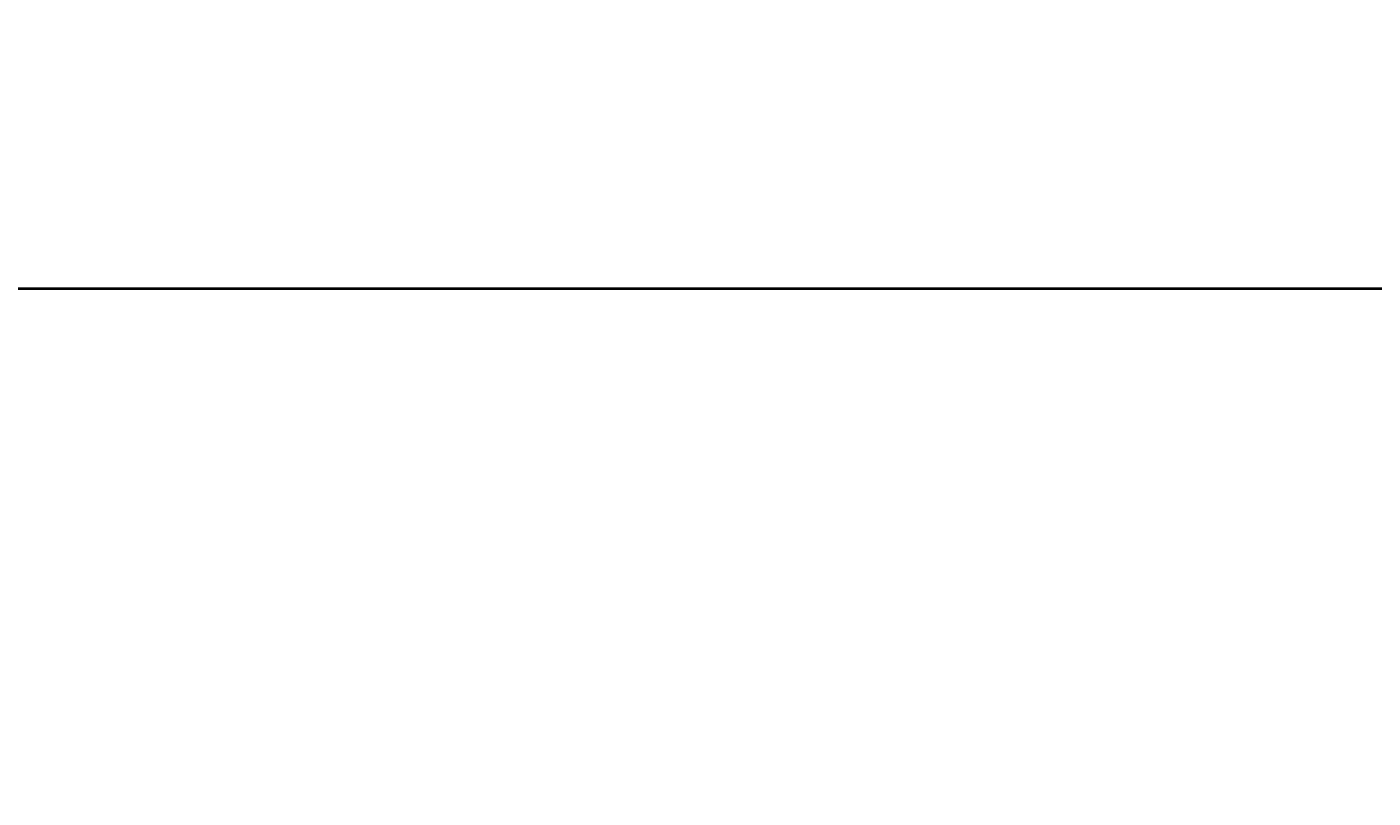
# Model space of a CAD drawing. Units: inches. Extents: x -301 to 715, y -607 to 364.
# Tile 63 of 141: x -93 to -62, y -235 to -218. Entities that reach past the tile are written whole.
import ezdxf

# ---------------------------------------------------------------- set-up
doc = ezdxf.new("R2010")
doc.units = ezdxf.units.IN
doc.header["$MEASUREMENT"] = 0
doc.layers.add('A-ANNO-DIMS', color=2, linetype='Continuous', lineweight=18)
doc.layers.add('A-WALL', color=3, linetype='Continuous', lineweight=40)
doc.styles.get("Standard").update_dxf_attribs({"font": 'arial.ttf'})
doc.dimstyles.get("Standard").update_dxf_attribs({"dimtxt": 0.18, "dimasz": 0.18, "dimexe": 0.18, "dimexo": 0.0625, "dimgap": 0.09, "dimtad": 0, "dimtih": 1, "dimtoh": 1, "dimdec": 1, "dimzin": 0, "dimdsep": 46, "dimlunit": 4, "dimtxsty": 'Standard', "dimcen": 0.09, "dimclrd": 3, "dimclre": 4, "dimclrt": 6, "dimadec": 0, "dimazin": 0, "dimtfac": 1, "dimtdec": 1, "dimtofl": 0, "dimtmove": 0, "dimatfit": 3, "dimfxl": 1, "dimtfill": 2, "dimtfillclr": 51, "dimtolj": 1, "dimtzin": 0, "dimarcsym": 0})

# ---------------------------------------------------------------- blocks, each defined once
blk = doc.blocks.new('*D147')
at = {"layer": 'A-ANNO-DIMS', "color": 4, "lineweight": -2, "transparency": 16777216}
for p, q in [((-103.603, -223.88), (-103.603, -296.865)), ((-45.603, -223.88), (-45.603, -296.865))]:
    blk.add_line(p, q, dxfattribs=at)
at = {"layer": 'A-ANNO-DIMS', "color": 3, "lineweight": -2, "transparency": 16777216}
for p, q in [((-103.423, -296.685), (-75.006, -296.685)), ((-45.783, -296.685), (-74.2, -296.685))]:
    blk.add_line(p, q, dxfattribs=at)
at = {"layer": 'A-ANNO-DIMS', "color": 3, "transparency": 16777216}
for points in [[(-103.423, -296.655), (-103.423, -296.715), (-103.603, -296.685)], [(-45.783, -296.655), (-45.783, -296.715), (-45.603, -296.685)]]:
    blk.add_solid(points, dxfattribs=at)
at = {"layer": 'Defpoints', "color": 0, "transparency": 16777216}
for p in [(-103.603, -223.818), (-45.603, -223.818), (-45.603, -296.685)]:
    blk.add_point(p, dxfattribs=at)
at = {"layer": 'A-ANNO-DIMS', "color": 6, "transparency": 16777216, "insert": (-74.603, -296.685), "char_height": 0.18, "attachment_point": 5, "bg_fill": 1, "box_fill_scale": 1.25, "bg_fill_color": 51, "bg_fill_transparency": 0}
blk.add_mtext('\\A1;4\'-10"', dxfattribs=at)
blk = doc.blocks.new('*D151')
at = {"layer": 'A-ANNO-DIMS', "color": 4, "lineweight": -2, "transparency": 16777216}
for p, q in [((-204.603, -223.755), (-204.603, 359.612)), ((-45.603, -214.755), (-45.603, 359.612))]:
    blk.add_line(p, q, dxfattribs=at)
at = {"layer": 'A-ANNO-DIMS', "color": 3, "lineweight": -2, "transparency": 16777216}
for p, q in [((-204.423, 359.432), (-125.494, 359.432)), ((-45.783, 359.432), (-124.713, 359.432))]:
    blk.add_line(p, q, dxfattribs=at)
at = {"layer": 'A-ANNO-DIMS', "color": 3, "transparency": 16777216}
for points in [[(-204.423, 359.462), (-204.423, 359.402), (-204.603, 359.432)], [(-45.783, 359.462), (-45.783, 359.402), (-45.603, 359.432)]]:
    blk.add_solid(points, dxfattribs=at)
at = {"layer": 'Defpoints', "color": 0, "transparency": 16777216}
for p in [(-45.603, 359.432), (-45.603, -214.818), (-204.603, -223.818)]:
    blk.add_point(p, dxfattribs=at)
at = {"layer": 'A-ANNO-DIMS', "color": 6, "transparency": 16777216, "insert": (-125.103, 359.432), "char_height": 0.18, "attachment_point": 5, "bg_fill": 1, "box_fill_scale": 1.25, "bg_fill_color": 51, "bg_fill_transparency": 0}
blk.add_mtext('\\A1;13\'-3"', dxfattribs=at)
blk = doc.blocks.new('*D158')
at = {"layer": 'A-ANNO-DIMS', "color": 4, "lineweight": -2, "transparency": 16777216}
for p, q in [((-122.603, 221.62), (-122.603, -296.865)), ((-50.603, 221.62), (-50.603, -296.865))]:
    blk.add_line(p, q, dxfattribs=at)
at = {"layer": 'A-ANNO-DIMS', "color": 3, "lineweight": -2, "transparency": 16777216}
for p, q in [((-122.423, -296.685), (-86.933, -296.685)), ((-50.783, -296.685), (-86.274, -296.685))]:
    blk.add_line(p, q, dxfattribs=at)
at = {"layer": 'A-ANNO-DIMS', "color": 3, "transparency": 16777216}
for points in [[(-122.423, -296.655), (-122.423, -296.715), (-122.603, -296.685)], [(-50.783, -296.655), (-50.783, -296.715), (-50.603, -296.685)]]:
    blk.add_solid(points, dxfattribs=at)
at = {"layer": 'Defpoints', "color": 0, "transparency": 16777216}
for p in [(-122.603, 221.682), (-50.603, 221.682), (-50.603, -296.685)]:
    blk.add_point(p, dxfattribs=at)
at = {"layer": 'A-ANNO-DIMS', "color": 6, "transparency": 16777216, "insert": (-86.603, -296.685), "char_height": 0.18, "attachment_point": 5, "bg_fill": 1, "box_fill_scale": 1.25, "bg_fill_color": 51, "bg_fill_transparency": 0}
blk.add_mtext('\\A1;6\'-0"', dxfattribs=at)

msp = doc.modelspace()

# ---------------------------------------------------------------- linework, layer by layer
at = {"layer": 'A-WALL'}
msp.add_line((-204.603, -223.818), (-45.603, -223.818), dxfattribs=at)

# ---------------------------------------------------------------- dimensions: what is measured, and where the dimension line sits
at = {"layer": 'A-ANNO-DIMS'}
for base, p1, p2, picture, middle in [((-45.603, 359.432), (-204.603, -223.818), (-45.603, -214.818), '*D151', (-125.103, 359.432)), ((-50.603, -296.685), (-122.603, 221.682), (-50.603, 221.682), '*D158', (-86.603, -296.685)), ((-45.603, -296.685), (-103.603, -223.818), (-45.603, -223.818), '*D147', (-74.603, -296.685))]:
    dim = msp.add_linear_dim(base=base, p1=p1, p2=p2, dimstyle='Standard', override={"dimdec": 1, "dimlfac": 1, "dimrnd": 0, "dimzin": 1, "dimdsep": 46, "dimlunit": 4, "dimfrac": 2}, dxfattribs=at)
    dim.commit()
    dim.dimension.update_dxf_attribs({"geometry": picture, "text_midpoint": middle})

doc.saveas('drawing.dxf')
